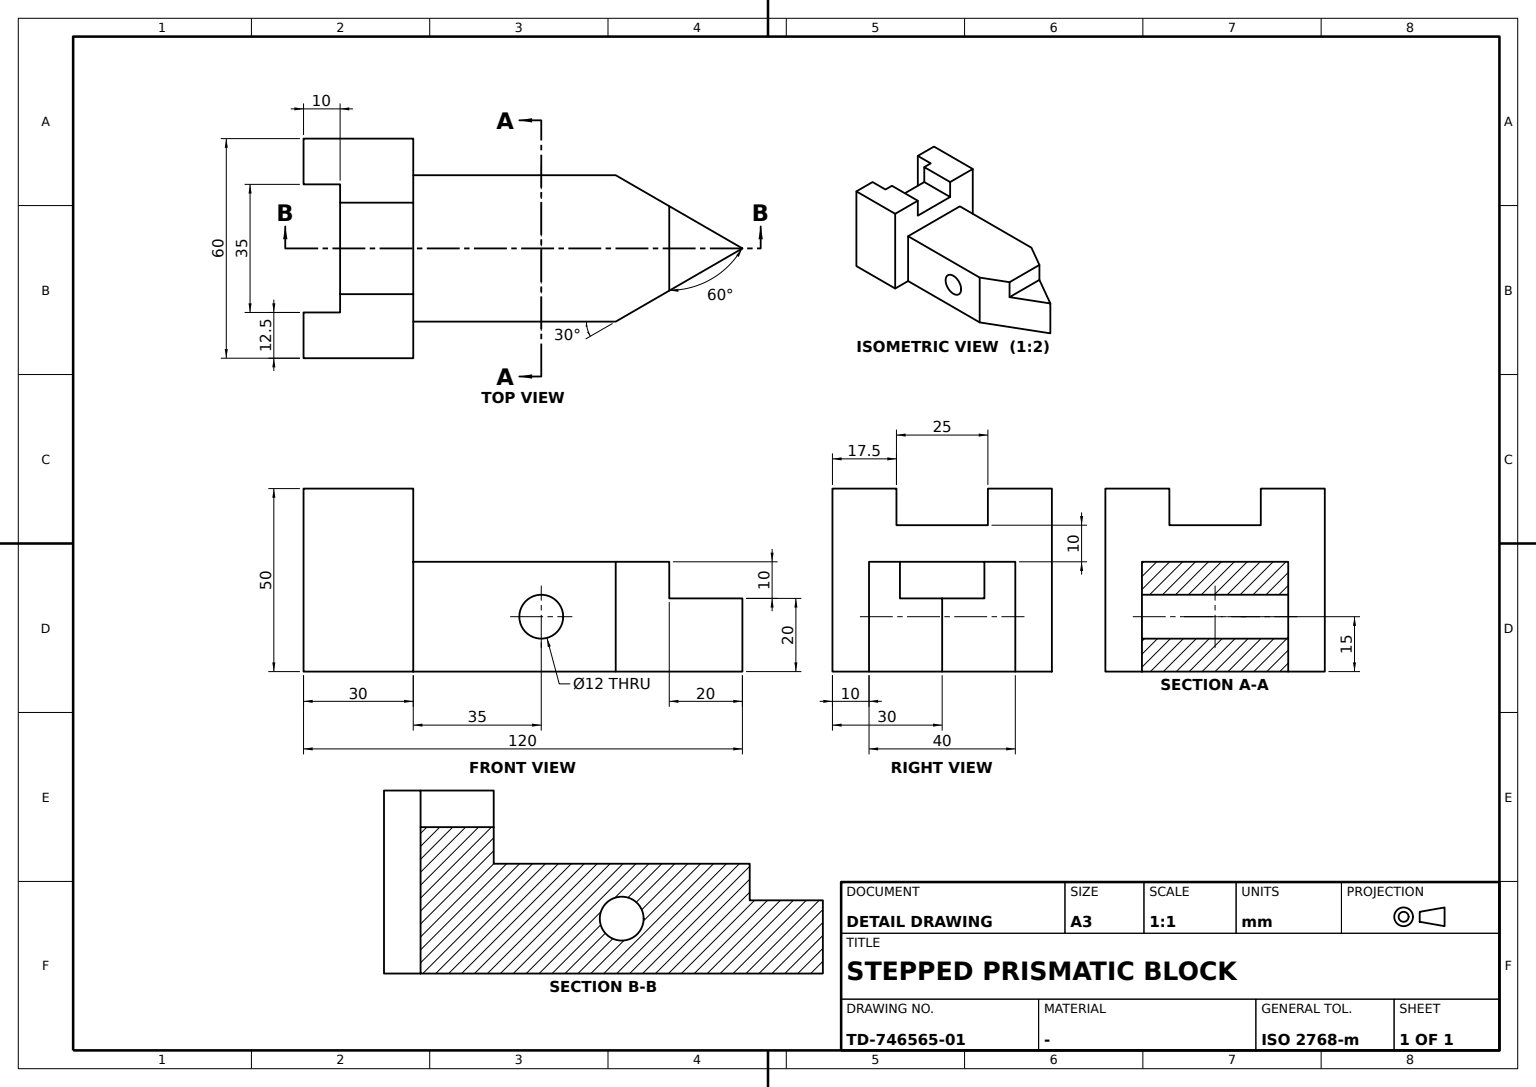
CATIA V5 part; units mm, degrees
sketch "Sketch1" plane through (0, 0, 0) normal (1, 0, 0) x (0, 1, 0)
  line L0 (0, 0) -> (0, 50)
  line L1 (0, 0) -> (120, 0)
  line L2 (0, 50) -> (30, 50)
  line L3 (120, 0) -> (120, 30)
  line L4 (30, 50) -> (30, 30)
  line L5 (30, 30) -> (120, 30)
  dimension "length L0" = 50
  dimension "length L1" = 120
  dimension "length L2" = 30
  dimension "length L3" = 30
  constraint vertical L0 y-axis
  constraint vertical L3 y-axis
  constraint vertical L4 y-axis
  constraint horizontal L1 x-axis
  constraint horizontal L2 x-axis
  constraint horizontal L5 x-axis
extrude "Pad1" add sketch "Sketch1" along normal mid plane 60
sketch "Sketch2" plane through (0, 0, 30) normal (0, 0, 1) x (1, 0, 0)
  line L0 (20, 120) -> (20, 30)
  point P0 (20, 120)
  point P1 (20, 30)
  line L1 (-30, 30) -> (30, 30) construction
  line L2 (-30, 120) -> (30, 120) construction
  line L3 (20, 120) -> (30, 120)
  line L4 (30, 120) -> (30, 30)
  line L5 (20, 30) -> (30, 30)
  line L6 (30, 120) -> (30, 30) construction
  dimension "distance L0 y axis" = 20
  constraint vertical L0 y-axis
  constraint vertical L4 y-axis
  constraint coincidence P1 L1
  constraint coincidence P0 L2
  constraint coincidence L4 L6
  constraint horizontal L3 x-axis
  constraint horizontal L5 x-axis
extrude "Pocket1" cut sketch "Sketch2" against normal blind 30
sketch "Sketch3" plane through (0, 0, 30) normal (0, 0, 1) x (1, 0, 0)
  line L0 (-30, 120) -> (-20, 120)
  line L1 (-20, 120) -> (-20, 30)
  line L2 (-20, 30) -> (-30, 30)
  line L3 (-30, 30) -> (-30, 120)
  line L4 (-30, 30) -> (30, 30) construction
  line L5 (-30, 120) -> (30, 120) construction
  line L6 (-30, 120) -> (-30, 30) construction
  dimension "distance L1 y axis" = 20
  constraint horizontal L0 x-axis
  constraint horizontal L2 x-axis
  constraint vertical L1 y-axis
  constraint vertical L3 y-axis
  constraint coincidence L2 L4
  constraint coincidence L0 L5
  constraint coincidence L3 L6
extrude "Pocket2" cut sketch "Sketch3" against normal blind 30
sketch "Sketch4" plane through (0, 0, 30) normal (0, 0, 1) x (1, 0, 0)
  line L0 (0, 120) -> (30.7045, 66.8182)
  point P0 (0, 120)
  line L1 (-30, 120) -> (30, 120) construction
  line L2 (0, 120) -> (30.7045, 120)
  line L3 (30.7045, 120) -> (30.7045, 66.8182)
  dimension "distance P0 y axis" = 0
  dimension "angle L0 y axis" = 30
  dimension "length L3" = 53.1818
  constraint coincidence P0 L1
  constraint horizontal L2 x-axis
  constraint vertical L3 y-axis
extrude "Pocket3" cut sketch "Sketch4" against normal blind 30
sketch "Sketch5" plane through (0, 0, 30) normal (0, 0, 1) x (1, 0, 0)
  line L0 (0, 120) -> (-20, 85.359)
  point P0 (0, 120)
  point P1 (-20, 85.359)
  point P2 (0, 120)
  line L1 (-20, 30) -> (-20, 120) construction
  line L2 (0, 120) -> (-20, 120)
  line L3 (-20, 120) -> (-20, 85.359)
  dimension "angle L0 y axis" = 30
  constraint coincidence P0 y-axis
  constraint coincidence P0 P2
  constraint coincidence P1 L1
  constraint horizontal L2 x-axis
  constraint vertical L3 y-axis
extrude "Pocket4" cut sketch "Sketch5" against normal blind 30
sketch "Sketch6" plane through (0, 0, 0) normal (1, 0, 0) x (0, 1, 0)
  line L0 (100, 30) -> (120, 30)
  line L1 (120, 30) -> (120, 20)
  line L2 (120, 20) -> (100, 20)
  line L3 (100, 20) -> (100, 30)
  line L4 (120, 30) -> (85.359, 30) construction
  line L5 (120, 30) -> (120, 0) construction
  dimension "length L1" = 10
  dimension "length L0" = 20
  constraint horizontal L0 x-axis
  constraint horizontal L2 x-axis
  constraint vertical L1 y-axis
  constraint vertical L3 y-axis
  constraint coincidence L0 L4
  constraint coincidence L1 L5
extrude "Pocket5" cut sketch "Sketch6" along normal mid plane 60
sketch "Sketch7" plane through (20, 0, 0) normal (1, 0, 0) x (0, 1, 0)
  circle A0 centre (65, 15) radius 6
  point P0 (65, 15)
  line L0 (120, 0) -> (30, 0) construction
  line L1 (30, 30) -> (30, 50) construction
  dimension "distance P0 L0" = 15
  dimension "distance P0 L1" = 35
  dimension "radius A0" = 6
extrude "Pocket6" cut sketch "Sketch7" against normal through all
sketch "Sketch8" plane through (0, 30, 0) normal (0, 1, 0) x (-1, 0, 0)
  point P0 (0, 45)
  line L0 (12.5, 50) -> (12.5, 40)
  line L1 (12.5, 40) -> (-12.5, 40)
  line L2 (-12.5, 40) -> (-12.5, 50)
  line L3 (-12.5, 50) -> (12.5, 50)
  line L4 (30, 50) -> (-30, 50) construction
  dimension "length L0" = 10
  dimension "length L1" = 25
  constraint coincidence P0 y-axis
  constraint coincidence L3 L4
  constraint vertical L0 y-axis
  constraint vertical L2 y-axis
  constraint horizontal L1 x-axis
  constraint horizontal L3 x-axis
  constraint equidistance L0 L2 P0
  constraint equidistance L1 L3 P0
extrude "Pocket7" cut sketch "Sketch8" against normal through all
sketch "Sketch9" plane through (0, 0, 50) normal (0, 0, 1) x (1, 0, 0)
  point P0 (0, 5)
  line L0 (17.5, 10) -> (17.5, 0)
  line L1 (17.5, 0) -> (-17.5, 0)
  line L2 (-17.5, 0) -> (-17.5, 10)
  line L3 (-17.5, 10) -> (17.5, 10)
  line L4 (-30, 0) -> (30, 0) construction
  dimension "length L0" = 10
  dimension "length L3" = 35
  constraint coincidence P0 y-axis
  constraint coincidence L1 L4
  constraint vertical L0 y-axis
  constraint vertical L2 y-axis
  constraint horizontal L1 x-axis
  constraint horizontal L3 x-axis
  constraint equidistance L0 L2 P0
  constraint equidistance L1 L3 P0
extrude "Pocket8" cut sketch "Sketch9" against normal through all
